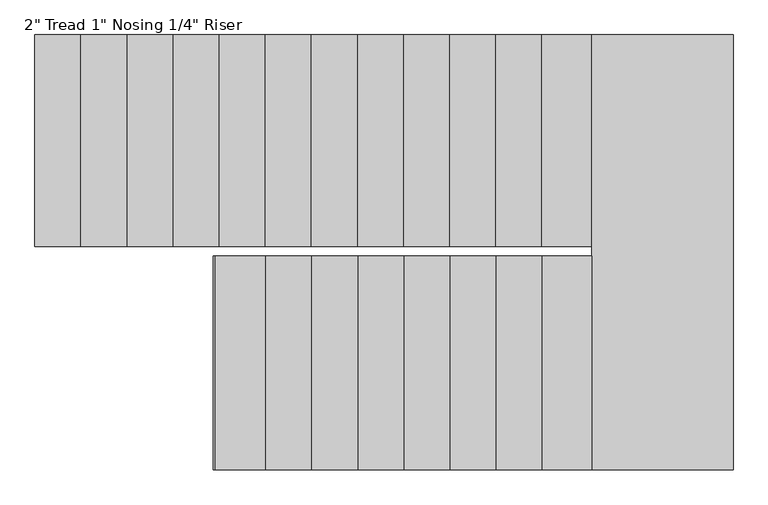
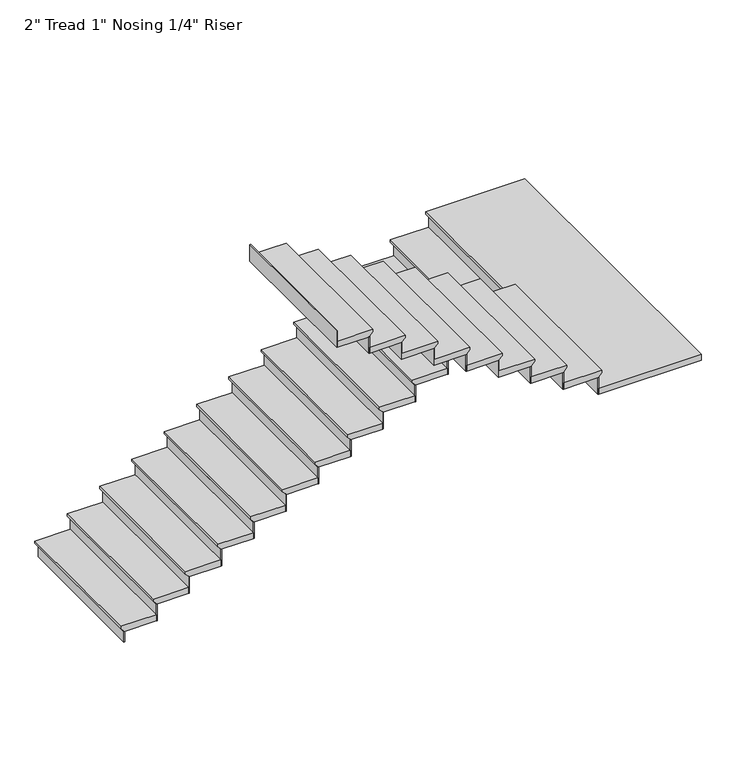
"""IFC4 building model written with IfcOpenShell, lengths in millimetres: stair flight geometry."""

from ifc_helpers import new_model, si_unit, origin, place, context, project, spatial, faceted_brep, source, transform, mapped, element, save


def stair_flight_e3e94c6b(model_context):
    return source(origin(), model_context, "Body", "Brep", [
        faceted_brep([(1811.8890963, 296.3962251, 3167.4954545), (1811.8890963, 296.3962251, 3186.5454545), (1811.8890963, 1464.7962251, 3186.5454545), (1811.8890963, 1464.7962251, 3167.4954545), (1837.2890963, 296.3962251, 3142.0954545), (1837.2890963, 1464.7962251, 3142.0954545), (2091.2890963, 296.3962251, 3186.5454545), (2091.2890963, 1464.7962251, 3186.5454545), (1837.2890963, 1464.7962251, 3135.7454545), (2091.2890963, 1464.7962251, 3135.7454545), (2091.2890963, 296.3962251, 3135.7454545), (1837.2890963, 296.3962251, 3135.7454545)], [[[0, 1, 2, 3]], [[4, 0, 3, 5]], [[2, 1, 6, 7]], [[8, 9, 10, 11]], [[2, 7, 9, 8, 5, 3]], [[8, 11, 4, 5]], [[6, 1, 0, 4, 11, 10]], [[7, 6, 10, 9]]]),
        faceted_brep([(1837.2890963, 296.3962251, 3135.7454545), (1837.2890963, 296.3962251, 3048.0), (1843.6390963, 296.3962251, 3048.0), (1843.6390963, 296.3962251, 3135.7454545), (1837.2890963, 1464.7962251, 3135.7454545), (1843.6390963, 1464.7962251, 3135.7454545), (1843.6390963, 1464.7962251, 3048.0), (1837.2890963, 1464.7962251, 3048.0)], [[[0, 1, 2, 3]], [[4, 5, 6, 7]], [[1, 0, 4, 7]], [[2, 1, 7, 6]], [[3, 2, 6, 5]], [[0, 3, 5, 4]]]),
        faceted_brep([(2091.2890963, 296.3962251, 3274.2909091), (2091.2890963, 296.3962251, 3135.7454545), (2097.6390963, 296.3962251, 3135.7454545), (2097.6390963, 296.3962251, 3274.2909091), (2091.2890963, 1464.7962251, 3274.2909091), (2097.6390963, 1464.7962251, 3274.2909091), (2097.6390963, 1464.7962251, 3135.7454545), (2091.2890963, 1464.7962251, 3135.7454545)], [[[0, 1, 2, 3]], [[4, 5, 6, 7]], [[1, 0, 4, 7]], [[2, 1, 7, 6]], [[3, 2, 6, 5]], [[0, 3, 5, 4]]]),
        faceted_brep([(2065.8890963, 1464.7962251, 3325.0909091), (2065.8890963, 296.3962251, 3325.0909091), (2345.2890963, 296.3962251, 3325.0909091), (2345.2890963, 1464.7962251, 3325.0909091), (2091.2890963, 1464.7962251, 3274.2909091), (2345.2890963, 1464.7962251, 3274.2909091), (2345.2890963, 296.3962251, 3274.2909091), (2091.2890963, 296.3962251, 3274.2909091), (2091.2890963, 1464.7962251, 3280.6409091), (2065.8890963, 1464.7962251, 3306.0409091), (2091.2890963, 296.3962251, 3280.6409091), (2065.8890963, 296.3962251, 3306.0409091)], [[[0, 1, 2, 3]], [[4, 5, 6, 7]], [[0, 3, 5, 4, 8, 9]], [[4, 7, 10, 8]], [[2, 1, 11, 10, 7, 6]], [[3, 2, 6, 5]], [[11, 1, 0, 9]], [[10, 11, 9, 8]]]),
        faceted_brep([(2345.2890963, 296.3962251, 3412.8363636), (2345.2890963, 296.3962251, 3274.2909091), (2351.6390963, 296.3962251, 3274.2909091), (2351.6390963, 296.3962251, 3412.8363636), (2345.2890963, 1464.7962251, 3412.8363636), (2351.6390963, 1464.7962251, 3412.8363636), (2351.6390963, 1464.7962251, 3274.2909091), (2345.2890963, 1464.7962251, 3274.2909091)], [[[0, 1, 2, 3]], [[4, 5, 6, 7]], [[1, 0, 4, 7]], [[2, 1, 7, 6]], [[3, 2, 6, 5]], [[0, 3, 5, 4]]]),
        faceted_brep([(2319.8890963, 1464.7962251, 3463.6363636), (2319.8890963, 296.3962251, 3463.6363636), (2599.2890963, 296.3962251, 3463.6363636), (2599.2890963, 1464.7962251, 3463.6363636), (2345.2890963, 1464.7962251, 3412.8363636), (2599.2890963, 1464.7962251, 3412.8363636), (2599.2890963, 296.3962251, 3412.8363636), (2345.2890963, 296.3962251, 3412.8363636), (2345.2890963, 1464.7962251, 3419.1863636), (2319.8890963, 1464.7962251, 3444.5863636), (2345.2890963, 296.3962251, 3419.1863636), (2319.8890963, 296.3962251, 3444.5863636)], [[[0, 1, 2, 3]], [[4, 5, 6, 7]], [[0, 3, 5, 4, 8, 9]], [[4, 7, 10, 8]], [[2, 1, 11, 10, 7, 6]], [[3, 2, 6, 5]], [[11, 1, 0, 9]], [[10, 11, 9, 8]]]),
        faceted_brep([(2599.2890963, 296.3962251, 3551.3818182), (2599.2890963, 296.3962251, 3412.8363636), (2605.6390963, 296.3962251, 3412.8363636), (2605.6390963, 296.3962251, 3551.3818182), (2599.2890963, 1464.7962251, 3551.3818182), (2605.6390963, 1464.7962251, 3551.3818182), (2605.6390963, 1464.7962251, 3412.8363636), (2599.2890963, 1464.7962251, 3412.8363636)], [[[0, 1, 2, 3]], [[4, 5, 6, 7]], [[1, 0, 4, 7]], [[2, 1, 7, 6]], [[3, 2, 6, 5]], [[0, 3, 5, 4]]]),
        faceted_brep([(2573.8890963, 1464.7962251, 3602.1818182), (2573.8890963, 296.3962251, 3602.1818182), (2853.2890963, 296.3962251, 3602.1818182), (2853.2890963, 1464.7962251, 3602.1818182), (2599.2890963, 1464.7962251, 3551.3818182), (2853.2890963, 1464.7962251, 3551.3818182), (2853.2890963, 296.3962251, 3551.3818182), (2599.2890963, 296.3962251, 3551.3818182), (2599.2890963, 1464.7962251, 3557.7318182), (2573.8890963, 1464.7962251, 3583.1318182), (2599.2890963, 296.3962251, 3557.7318182), (2573.8890963, 296.3962251, 3583.1318182)], [[[0, 1, 2, 3]], [[4, 5, 6, 7]], [[0, 3, 5, 4, 8, 9]], [[4, 7, 10, 8]], [[2, 1, 11, 10, 7, 6]], [[3, 2, 6, 5]], [[11, 1, 0, 9]], [[10, 11, 9, 8]]]),
        faceted_brep([(2853.2890963, 296.3962251, 3689.9272727), (2853.2890963, 296.3962251, 3551.3818182), (2859.6390963, 296.3962251, 3551.3818182), (2859.6390963, 296.3962251, 3689.9272727), (2853.2890963, 1464.7962251, 3689.9272727), (2859.6390963, 1464.7962251, 3689.9272727), (2859.6390963, 1464.7962251, 3551.3818182), (2853.2890963, 1464.7962251, 3551.3818182)], [[[0, 1, 2, 3]], [[4, 5, 6, 7]], [[1, 0, 4, 7]], [[2, 1, 7, 6]], [[3, 2, 6, 5]], [[0, 3, 5, 4]]]),
        faceted_brep([(2827.8890963, 1464.7962251, 3740.7272727), (2827.8890963, 296.3962251, 3740.7272727), (3107.2890963, 296.3962251, 3740.7272727), (3107.2890963, 1464.7962251, 3740.7272727), (2853.2890963, 1464.7962251, 3689.9272727), (3107.2890963, 1464.7962251, 3689.9272727), (3107.2890963, 296.3962251, 3689.9272727), (2853.2890963, 296.3962251, 3689.9272727), (2853.2890963, 1464.7962251, 3696.2772727), (2827.8890963, 1464.7962251, 3721.6772727), (2853.2890963, 296.3962251, 3696.2772727), (2827.8890963, 296.3962251, 3721.6772727)], [[[0, 1, 2, 3]], [[4, 5, 6, 7]], [[0, 3, 5, 4, 8, 9]], [[4, 7, 10, 8]], [[2, 1, 11, 10, 7, 6]], [[3, 2, 6, 5]], [[11, 1, 0, 9]], [[10, 11, 9, 8]]]),
        faceted_brep([(3107.2890963, 296.3962251, 3828.4727273), (3107.2890963, 296.3962251, 3689.9272727), (3113.6390963, 296.3962251, 3689.9272727), (3113.6390963, 296.3962251, 3828.4727273), (3107.2890963, 1464.7962251, 3828.4727273), (3113.6390963, 1464.7962251, 3828.4727273), (3113.6390963, 1464.7962251, 3689.9272727), (3107.2890963, 1464.7962251, 3689.9272727)], [[[0, 1, 2, 3]], [[4, 5, 6, 7]], [[1, 0, 4, 7]], [[2, 1, 7, 6]], [[3, 2, 6, 5]], [[0, 3, 5, 4]]]),
        faceted_brep([(3081.8890963, 1464.7962251, 3879.2727273), (3081.8890963, 296.3962251, 3879.2727273), (3361.2890963, 296.3962251, 3879.2727273), (3361.2890963, 1464.7962251, 3879.2727273), (3107.2890963, 1464.7962251, 3828.4727273), (3361.2890963, 1464.7962251, 3828.4727273), (3361.2890963, 296.3962251, 3828.4727273), (3107.2890963, 296.3962251, 3828.4727273), (3107.2890963, 1464.7962251, 3834.8227273), (3081.8890963, 1464.7962251, 3860.2227273), (3107.2890963, 296.3962251, 3834.8227273), (3081.8890963, 296.3962251, 3860.2227273)], [[[0, 1, 2, 3]], [[4, 5, 6, 7]], [[0, 3, 5, 4, 8, 9]], [[4, 7, 10, 8]], [[2, 1, 11, 10, 7, 6]], [[3, 2, 6, 5]], [[11, 1, 0, 9]], [[10, 11, 9, 8]]]),
        faceted_brep([(3361.2890963, 296.3962251, 3967.0181818), (3361.2890963, 296.3962251, 3828.4727273), (3367.6390963, 296.3962251, 3828.4727273), (3367.6390963, 296.3962251, 3967.0181818), (3361.2890963, 1464.7962251, 3967.0181818), (3367.6390963, 1464.7962251, 3967.0181818), (3367.6390963, 1464.7962251, 3828.4727273), (3361.2890963, 1464.7962251, 3828.4727273)], [[[0, 1, 2, 3]], [[4, 5, 6, 7]], [[1, 0, 4, 7]], [[2, 1, 7, 6]], [[3, 2, 6, 5]], [[0, 3, 5, 4]]]),
        faceted_brep([(3335.8890963, 1464.7962251, 4017.8181818), (3335.8890963, 296.3962251, 4017.8181818), (3615.2890963, 296.3962251, 4017.8181818), (3615.2890963, 1464.7962251, 4017.8181818), (3361.2890963, 1464.7962251, 3967.0181818), (3615.2890963, 1464.7962251, 3967.0181818), (3615.2890963, 296.3962251, 3967.0181818), (3361.2890963, 296.3962251, 3967.0181818), (3361.2890963, 1464.7962251, 3973.3681818), (3335.8890963, 1464.7962251, 3998.7681818), (3361.2890963, 296.3962251, 3973.3681818), (3335.8890963, 296.3962251, 3998.7681818)], [[[0, 1, 2, 3]], [[4, 5, 6, 7]], [[0, 3, 5, 4, 8, 9]], [[4, 7, 10, 8]], [[2, 1, 11, 10, 7, 6]], [[3, 2, 6, 5]], [[11, 1, 0, 9]], [[10, 11, 9, 8]]]),
        faceted_brep([(3615.2890963, 296.3962251, 4105.5636364), (3615.2890963, 296.3962251, 3967.0181818), (3621.6390963, 296.3962251, 3967.0181818), (3621.6390963, 296.3962251, 4105.5636364), (3615.2890963, 1464.7962251, 4105.5636364), (3621.6390963, 1464.7962251, 4105.5636364), (3621.6390963, 1464.7962251, 3967.0181818), (3615.2890963, 1464.7962251, 3967.0181818)], [[[0, 1, 2, 3]], [[4, 5, 6, 7]], [[1, 0, 4, 7]], [[2, 1, 7, 6]], [[3, 2, 6, 5]], [[0, 3, 5, 4]]]),
        faceted_brep([(3589.8890963, 1464.7962251, 4156.3636364), (3589.8890963, 296.3962251, 4156.3636364), (3869.2890963, 296.3962251, 4156.3636364), (3869.2890963, 1464.7962251, 4156.3636364), (3615.2890963, 1464.7962251, 4105.5636364), (3869.2890963, 1464.7962251, 4105.5636364), (3869.2890963, 296.3962251, 4105.5636364), (3615.2890963, 296.3962251, 4105.5636364), (3615.2890963, 1464.7962251, 4111.9136364), (3589.8890963, 1464.7962251, 4137.3136364), (3615.2890963, 296.3962251, 4111.9136364), (3589.8890963, 296.3962251, 4137.3136364)], [[[0, 1, 2, 3]], [[4, 5, 6, 7]], [[0, 3, 5, 4, 8, 9]], [[4, 7, 10, 8]], [[2, 1, 11, 10, 7, 6]], [[3, 2, 6, 5]], [[11, 1, 0, 9]], [[10, 11, 9, 8]]]),
        faceted_brep([(3869.2890963, 296.3962251, 4244.1090909), (3869.2890963, 296.3962251, 4105.5636364), (3875.6390963, 296.3962251, 4105.5636364), (3875.6390963, 296.3962251, 4244.1090909), (3869.2890963, 1464.7962251, 4244.1090909), (3875.6390963, 1464.7962251, 4244.1090909), (3875.6390963, 1464.7962251, 4105.5636364), (3869.2890963, 1464.7962251, 4105.5636364)], [[[0, 1, 2, 3]], [[4, 5, 6, 7]], [[1, 0, 4, 7]], [[2, 1, 7, 6]], [[3, 2, 6, 5]], [[0, 3, 5, 4]]]),
        faceted_brep([(3843.8890963, 1464.7962251, 4294.9090909), (3843.8890963, 296.3962251, 4294.9090909), (4123.2890963, 296.3962251, 4294.9090909), (4123.2890963, 1464.7962251, 4294.9090909), (3869.2890963, 1464.7962251, 4244.1090909), (4123.2890963, 1464.7962251, 4244.1090909), (4123.2890963, 296.3962251, 4244.1090909), (3869.2890963, 296.3962251, 4244.1090909), (3869.2890963, 1464.7962251, 4250.4590909), (3843.8890963, 1464.7962251, 4275.8590909), (3869.2890963, 296.3962251, 4250.4590909), (3843.8890963, 296.3962251, 4275.8590909)], [[[0, 1, 2, 3]], [[4, 5, 6, 7]], [[0, 3, 5, 4, 8, 9]], [[4, 7, 10, 8]], [[2, 1, 11, 10, 7, 6]], [[3, 2, 6, 5]], [[11, 1, 0, 9]], [[10, 11, 9, 8]]]),
        faceted_brep([(4123.2890963, 296.3962251, 4382.6545455), (4123.2890963, 296.3962251, 4244.1090909), (4129.6390963, 296.3962251, 4244.1090909), (4129.6390963, 296.3962251, 4382.6545455), (4123.2890963, 1464.7962251, 4382.6545455), (4129.6390963, 1464.7962251, 4382.6545455), (4129.6390963, 1464.7962251, 4244.1090909), (4123.2890963, 1464.7962251, 4244.1090909)], [[[0, 1, 2, 3]], [[4, 5, 6, 7]], [[1, 0, 4, 7]], [[2, 1, 7, 6]], [[3, 2, 6, 5]], [[0, 3, 5, 4]]]),
        faceted_brep([(4097.8890963, 1464.7962251, 4433.4545455), (4097.8890963, 296.3962251, 4433.4545455), (4377.2890963, 296.3962251, 4433.4545455), (4377.2890963, 1464.7962251, 4433.4545455), (4123.2890963, 1464.7962251, 4382.6545455), (4377.2890963, 1464.7962251, 4382.6545455), (4377.2890963, 296.3962251, 4382.6545455), (4123.2890963, 296.3962251, 4382.6545455), (4123.2890963, 1464.7962251, 4389.0045455), (4097.8890963, 1464.7962251, 4414.4045455), (4123.2890963, 296.3962251, 4389.0045455), (4097.8890963, 296.3962251, 4414.4045455)], [[[0, 1, 2, 3]], [[4, 5, 6, 7]], [[0, 3, 5, 4, 8, 9]], [[4, 7, 10, 8]], [[2, 1, 11, 10, 7, 6]], [[3, 2, 6, 5]], [[11, 1, 0, 9]], [[10, 11, 9, 8]]]),
        faceted_brep([(4377.2890963, 296.3962251, 4521.2), (4377.2890963, 296.3962251, 4382.6545455), (4383.6390963, 296.3962251, 4382.6545455), (4383.6390963, 296.3962251, 4521.2), (4377.2890963, 1464.7962251, 4521.2), (4383.6390963, 1464.7962251, 4521.2), (4383.6390963, 1464.7962251, 4382.6545455), (4377.2890963, 1464.7962251, 4382.6545455)], [[[0, 1, 2, 3]], [[4, 5, 6, 7]], [[1, 0, 4, 7]], [[2, 1, 7, 6]], [[3, 2, 6, 5]], [[0, 3, 5, 4]]]),
        faceted_brep([(4351.8890963, 1464.7962251, 4572.0), (4351.8890963, 296.3962251, 4572.0), (4631.2890963, 296.3962251, 4572.0), (4631.2890963, 1464.7962251, 4572.0), (4377.2890963, 1464.7962251, 4521.2), (4631.2890963, 1464.7962251, 4521.2), (4631.2890963, 296.3962251, 4521.2), (4377.2890963, 296.3962251, 4521.2), (4377.2890963, 1464.7962251, 4527.55), (4351.8890963, 1464.7962251, 4552.95), (4377.2890963, 296.3962251, 4527.55), (4351.8890963, 296.3962251, 4552.95)], [[[0, 1, 2, 3]], [[4, 5, 6, 7]], [[0, 3, 5, 4, 8, 9]], [[4, 7, 10, 8]], [[2, 1, 11, 10, 7, 6]], [[3, 2, 6, 5]], [[11, 1, 0, 9]], [[10, 11, 9, 8]]]),
        faceted_brep([(4631.2890963, 296.3962251, 4659.7454545), (4631.2890963, 296.3962251, 4521.2), (4637.6390963, 296.3962251, 4521.2), (4637.6390963, 296.3962251, 4659.7454545), (4631.2890963, 1464.7962251, 4659.7454545), (4637.6390963, 1464.7962251, 4659.7454545), (4637.6390963, 1464.7962251, 4521.2), (4631.2890963, 1464.7962251, 4521.2)], [[[0, 1, 2, 3]], [[4, 5, 6, 7]], [[1, 0, 4, 7]], [[2, 1, 7, 6]], [[3, 2, 6, 5]], [[0, 3, 5, 4]]]),
        faceted_brep([(4605.8890963, 1464.7962251, 4710.5454545), (4605.8890963, 296.3962251, 4710.5454545), (4906.4326586, 296.3962251, 4710.5454545), (4906.4326586, 1464.7962251, 4710.5454545), (4631.2890963, 1464.7962251, 4659.7454545), (4906.4326586, 1464.7962251, 4659.7454545), (4906.4326586, 296.3962251, 4659.7454545), (4631.2890963, 296.3962251, 4659.7454545), (4631.2890963, 1464.7962251, 4666.0954545), (4605.8890963, 1464.7962251, 4691.4954545), (4631.2890963, 296.3962251, 4666.0954545), (4605.8890963, 296.3962251, 4691.4954545)], [[[0, 1, 2, 3]], [[4, 5, 6, 7]], [[0, 3, 5, 4, 8, 9]], [[4, 7, 10, 8]], [[2, 1, 11, 10, 7, 6]], [[3, 2, 6, 5]], [[11, 1, 0, 9]], [[10, 11, 9, 8]]]),
        faceted_brep([(4906.4326586, 296.3962251, 4798.2909091), (4906.4326586, 296.3962251, 4659.7454545), (4912.7826586, 296.3962251, 4659.7454545), (4912.7826586, 296.3962251, 4798.2909091), (4906.4326586, 1464.7962251, 4798.2909091), (4912.7826586, 1464.7962251, 4798.2909091), (4912.7826586, 1464.7962251, 4659.7454545), (4906.4326586, 1464.7962251, 4659.7454545)], [[[0, 1, 2, 3]], [[4, 5, 6, 7]], [[1, 0, 4, 7]], [[2, 1, 7, 6]], [[3, 2, 6, 5]], [[0, 3, 5, 4]]]),
        faceted_brep([(4855.6326586, -935.5037749, 4849.0909091), (5659.9890963, -935.5037749, 4849.0909091), (5659.9890963, 1464.7962251, 4849.0909091), (4881.0326586, 1464.7962251, 4849.0909091), (4881.0326586, 245.5962251, 4849.0909091), (4855.6326586, 245.5962251, 4849.0909091), (5659.9890963, -935.5037749, 4798.2909091), (4855.6326586, -935.5037749, 4798.2909091), (4855.6326586, 245.5962251, 4798.2909091), (4881.0326586, 245.5962251, 4798.2909091), (4881.0326586, 296.3962251, 4798.2909091), (4906.4326586, 296.3962251, 4798.2909091), (4906.4326586, 1464.7962251, 4798.2909091), (5659.9890963, 1464.7962251, 4798.2909091), (4906.4326586, 1464.7962251, 4804.6409091), (4881.0326586, 1464.7962251, 4830.0409091), (4906.4326586, 296.3962251, 4804.6409091), (4881.0326586, 296.3962251, 4830.0409091)], [[[0, 1, 2, 3, 4, 5]], [[6, 7, 8, 9, 10, 11, 12, 13]], [[1, 0, 7, 6]], [[2, 1, 6, 13]], [[3, 2, 13, 12, 14, 15]], [[12, 11, 16, 14]], [[11, 10, 17, 16]], [[4, 3, 15, 17, 10, 9]], [[5, 4, 9, 8]], [[0, 5, 8, 7]], [[15, 14, 16, 17]]]),
        faceted_brep([(4855.6326586, 245.5962251, 4936.8363636), (4855.6326586, 245.5962251, 4798.2909091), (4849.2826586, 245.5962251, 4798.2909091), (4849.2826586, 245.5962251, 4936.8363636), (4855.6326586, -935.5037749, 4936.8363636), (4849.2826586, -935.5037749, 4936.8363636), (4849.2826586, -935.5037749, 4798.2909091), (4855.6326586, -935.5037749, 4798.2909091)], [[[0, 1, 2, 3]], [[4, 5, 6, 7]], [[1, 0, 4, 7]], [[2, 1, 7, 6]], [[3, 2, 6, 5]], [[0, 3, 5, 4]]]),
        faceted_brep([(4881.0326586, -935.5037749, 4987.6363636), (4881.0326586, 245.5962251, 4987.6363636), (4580.4890963, 245.5962251, 4987.6363636), (4580.4890963, -935.5037749, 4987.6363636), (4855.6326586, -935.5037749, 4936.8363636), (4580.4890963, -935.5037749, 4936.8363636), (4580.4890963, 245.5962251, 4936.8363636), (4855.6326586, 245.5962251, 4936.8363636), (4855.6326586, -935.5037749, 4943.1863636), (4881.0326586, -935.5037749, 4968.5863636), (4855.6326586, 245.5962251, 4943.1863636), (4881.0326586, 245.5962251, 4968.5863636)], [[[0, 1, 2, 3]], [[4, 5, 6, 7]], [[0, 3, 5, 4, 8, 9]], [[4, 7, 10, 8]], [[2, 1, 11, 10, 7, 6]], [[3, 2, 6, 5]], [[11, 1, 0, 9]], [[10, 11, 9, 8]]]),
        faceted_brep([(4580.4890963, 245.5962251, 5075.3818182), (4580.4890963, 245.5962251, 4936.8363636), (4574.1390963, 245.5962251, 4936.8363636), (4574.1390963, 245.5962251, 5075.3818182), (4580.4890963, -935.5037749, 5075.3818182), (4574.1390963, -935.5037749, 5075.3818182), (4574.1390963, -935.5037749, 4936.8363636), (4580.4890963, -935.5037749, 4936.8363636)], [[[0, 1, 2, 3]], [[4, 5, 6, 7]], [[1, 0, 4, 7]], [[2, 1, 7, 6]], [[3, 2, 6, 5]], [[0, 3, 5, 4]]]),
        faceted_brep([(4605.8890963, -935.5037749, 5126.1818182), (4605.8890963, 245.5962251, 5126.1818182), (4326.4890963, 245.5962251, 5126.1818182), (4326.4890963, -935.5037749, 5126.1818182), (4580.4890963, -935.5037749, 5075.3818182), (4326.4890963, -935.5037749, 5075.3818182), (4326.4890963, 245.5962251, 5075.3818182), (4580.4890963, 245.5962251, 5075.3818182), (4580.4890963, -935.5037749, 5081.7318182), (4605.8890963, -935.5037749, 5107.1318182), (4580.4890963, 245.5962251, 5081.7318182), (4605.8890963, 245.5962251, 5107.1318182)], [[[0, 1, 2, 3]], [[4, 5, 6, 7]], [[0, 3, 5, 4, 8, 9]], [[4, 7, 10, 8]], [[2, 1, 11, 10, 7, 6]], [[3, 2, 6, 5]], [[11, 1, 0, 9]], [[10, 11, 9, 8]]]),
        faceted_brep([(4326.4890963, 245.5962251, 5213.9272727), (4326.4890963, 245.5962251, 5075.3818182), (4320.1390963, 245.5962251, 5075.3818182), (4320.1390963, 245.5962251, 5213.9272727), (4326.4890963, -935.5037749, 5213.9272727), (4320.1390963, -935.5037749, 5213.9272727), (4320.1390963, -935.5037749, 5075.3818182), (4326.4890963, -935.5037749, 5075.3818182)], [[[0, 1, 2, 3]], [[4, 5, 6, 7]], [[1, 0, 4, 7]], [[2, 1, 7, 6]], [[3, 2, 6, 5]], [[0, 3, 5, 4]]]),
        faceted_brep([(4351.8890963, -935.5037749, 5264.7272727), (4351.8890963, 245.5962251, 5264.7272727), (4072.4890963, 245.5962251, 5264.7272727), (4072.4890963, -935.5037749, 5264.7272727), (4326.4890963, -935.5037749, 5213.9272727), (4072.4890963, -935.5037749, 5213.9272727), (4072.4890963, 245.5962251, 5213.9272727), (4326.4890963, 245.5962251, 5213.9272727), (4326.4890963, -935.5037749, 5220.2772727), (4351.8890963, -935.5037749, 5245.6772727), (4326.4890963, 245.5962251, 5220.2772727), (4351.8890963, 245.5962251, 5245.6772727)], [[[0, 1, 2, 3]], [[4, 5, 6, 7]], [[0, 3, 5, 4, 8, 9]], [[4, 7, 10, 8]], [[2, 1, 11, 10, 7, 6]], [[3, 2, 6, 5]], [[11, 1, 0, 9]], [[10, 11, 9, 8]]]),
        faceted_brep([(4072.4890963, 245.5962251, 5352.4727273), (4072.4890963, 245.5962251, 5213.9272727), (4066.1390963, 245.5962251, 5213.9272727), (4066.1390963, 245.5962251, 5352.4727273), (4072.4890963, -935.5037749, 5352.4727273), (4066.1390963, -935.5037749, 5352.4727273), (4066.1390963, -935.5037749, 5213.9272727), (4072.4890963, -935.5037749, 5213.9272727)], [[[0, 1, 2, 3]], [[4, 5, 6, 7]], [[1, 0, 4, 7]], [[2, 1, 7, 6]], [[3, 2, 6, 5]], [[0, 3, 5, 4]]]),
        faceted_brep([(4097.8890963, -935.5037749, 5403.2727273), (4097.8890963, 245.5962251, 5403.2727273), (3818.4890963, 245.5962251, 5403.2727273), (3818.4890963, -935.5037749, 5403.2727273), (4072.4890963, -935.5037749, 5352.4727273), (3818.4890963, -935.5037749, 5352.4727273), (3818.4890963, 245.5962251, 5352.4727273), (4072.4890963, 245.5962251, 5352.4727273), (4072.4890963, -935.5037749, 5358.8227273), (4097.8890963, -935.5037749, 5384.2227273), (4072.4890963, 245.5962251, 5358.8227273), (4097.8890963, 245.5962251, 5384.2227273)], [[[0, 1, 2, 3]], [[4, 5, 6, 7]], [[0, 3, 5, 4, 8, 9]], [[4, 7, 10, 8]], [[2, 1, 11, 10, 7, 6]], [[3, 2, 6, 5]], [[11, 1, 0, 9]], [[10, 11, 9, 8]]]),
        faceted_brep([(3818.4890963, 245.5962251, 5491.0181818), (3818.4890963, 245.5962251, 5352.4727273), (3812.1390963, 245.5962251, 5352.4727273), (3812.1390963, 245.5962251, 5491.0181818), (3818.4890963, -935.5037749, 5491.0181818), (3812.1390963, -935.5037749, 5491.0181818), (3812.1390963, -935.5037749, 5352.4727273), (3818.4890963, -935.5037749, 5352.4727273)], [[[0, 1, 2, 3]], [[4, 5, 6, 7]], [[1, 0, 4, 7]], [[2, 1, 7, 6]], [[3, 2, 6, 5]], [[0, 3, 5, 4]]]),
        faceted_brep([(3843.8890963, -935.5037749, 5541.8181818), (3843.8890963, 245.5962251, 5541.8181818), (3564.4890963, 245.5962251, 5541.8181818), (3564.4890963, -935.5037749, 5541.8181818), (3818.4890963, -935.5037749, 5491.0181818), (3564.4890963, -935.5037749, 5491.0181818), (3564.4890963, 245.5962251, 5491.0181818), (3818.4890963, 245.5962251, 5491.0181818), (3818.4890963, -935.5037749, 5497.3681818), (3843.8890963, -935.5037749, 5522.7681818), (3818.4890963, 245.5962251, 5497.3681818), (3843.8890963, 245.5962251, 5522.7681818)], [[[0, 1, 2, 3]], [[4, 5, 6, 7]], [[0, 3, 5, 4, 8, 9]], [[4, 7, 10, 8]], [[2, 1, 11, 10, 7, 6]], [[3, 2, 6, 5]], [[11, 1, 0, 9]], [[10, 11, 9, 8]]]),
        faceted_brep([(3564.4890963, 245.5962251, 5629.5636364), (3564.4890963, 245.5962251, 5491.0181818), (3558.1390963, 245.5962251, 5491.0181818), (3558.1390963, 245.5962251, 5629.5636364), (3564.4890963, -935.5037749, 5629.5636364), (3558.1390963, -935.5037749, 5629.5636364), (3558.1390963, -935.5037749, 5491.0181818), (3564.4890963, -935.5037749, 5491.0181818)], [[[0, 1, 2, 3]], [[4, 5, 6, 7]], [[1, 0, 4, 7]], [[2, 1, 7, 6]], [[3, 2, 6, 5]], [[0, 3, 5, 4]]]),
        faceted_brep([(3589.8890963, -935.5037749, 5680.3636364), (3589.8890963, 245.5962251, 5680.3636364), (3310.4890963, 245.5962251, 5680.3636364), (3310.4890963, -935.5037749, 5680.3636364), (3564.4890963, -935.5037749, 5629.5636364), (3310.4890963, -935.5037749, 5629.5636364), (3310.4890963, 245.5962251, 5629.5636364), (3564.4890963, 245.5962251, 5629.5636364), (3564.4890963, -935.5037749, 5635.9136364), (3589.8890963, -935.5037749, 5661.3136364), (3564.4890963, 245.5962251, 5635.9136364), (3589.8890963, 245.5962251, 5661.3136364)], [[[0, 1, 2, 3]], [[4, 5, 6, 7]], [[0, 3, 5, 4, 8, 9]], [[4, 7, 10, 8]], [[2, 1, 11, 10, 7, 6]], [[3, 2, 6, 5]], [[11, 1, 0, 9]], [[10, 11, 9, 8]]]),
        faceted_brep([(3310.4890963, 245.5962251, 5768.1090909), (3310.4890963, 245.5962251, 5629.5636364), (3304.1390963, 245.5962251, 5629.5636364), (3304.1390963, 245.5962251, 5768.1090909), (3310.4890963, -935.5037749, 5768.1090909), (3304.1390963, -935.5037749, 5768.1090909), (3304.1390963, -935.5037749, 5629.5636364), (3310.4890963, -935.5037749, 5629.5636364)], [[[0, 1, 2, 3]], [[4, 5, 6, 7]], [[1, 0, 4, 7]], [[2, 1, 7, 6]], [[3, 2, 6, 5]], [[0, 3, 5, 4]]]),
        faceted_brep([(3335.8890963, -935.5037749, 5818.9090909), (3335.8890963, 245.5962251, 5818.9090909), (3056.4890963, 245.5962251, 5818.9090909), (3056.4890963, -935.5037749, 5818.9090909), (3310.4890963, -935.5037749, 5768.1090909), (3056.4890963, -935.5037749, 5768.1090909), (3056.4890963, 245.5962251, 5768.1090909), (3310.4890963, 245.5962251, 5768.1090909), (3310.4890963, -935.5037749, 5774.4590909), (3335.8890963, -935.5037749, 5799.8590909), (3310.4890963, 245.5962251, 5774.4590909), (3335.8890963, 245.5962251, 5799.8590909)], [[[0, 1, 2, 3]], [[4, 5, 6, 7]], [[0, 3, 5, 4, 8, 9]], [[4, 7, 10, 8]], [[2, 1, 11, 10, 7, 6]], [[3, 2, 6, 5]], [[11, 1, 0, 9]], [[10, 11, 9, 8]]]),
        faceted_brep([(3056.4890963, 245.5962251, 5906.6545455), (3056.4890963, 245.5962251, 5768.1090909), (3050.1390963, 245.5962251, 5768.1090909), (3050.1390963, 245.5962251, 5906.6545455), (3056.4890963, -935.5037749, 5906.6545455), (3050.1390963, -935.5037749, 5906.6545455), (3050.1390963, -935.5037749, 5768.1090909), (3056.4890963, -935.5037749, 5768.1090909)], [[[0, 1, 2, 3]], [[4, 5, 6, 7]], [[1, 0, 4, 7]], [[2, 1, 7, 6]], [[3, 2, 6, 5]], [[0, 3, 5, 4]]]),
        faceted_brep([(2802.4890963, 245.5962251, 6045.2), (2802.4890963, 245.5962251, 5906.6545455), (2796.1390963, 245.5962251, 5906.6545455), (2796.1390963, 245.5962251, 6045.2), (2802.4890963, -935.5037749, 6045.2), (2796.1390963, -935.5037749, 6045.2), (2796.1390963, -935.5037749, 5906.6545455), (2802.4890963, -935.5037749, 5906.6545455)], [[[0, 1, 2, 3]], [[4, 5, 6, 7]], [[1, 0, 4, 7]], [[2, 1, 7, 6]], [[3, 2, 6, 5]], [[0, 3, 5, 4]]]),
        faceted_brep([(3081.8890963, -935.5037749, 5957.4545455), (3081.8890963, 245.5962251, 5957.4545455), (2802.4890963, 245.5962251, 5957.4545455), (2802.4890963, -935.5037749, 5957.4545455), (3056.4890963, -935.5037749, 5906.6545455), (2802.4890963, -935.5037749, 5906.6545455), (2802.4890963, 245.5962251, 5906.6545455), (3056.4890963, 245.5962251, 5906.6545455), (3056.4890963, -935.5037749, 5913.0045455), (3081.8890963, -935.5037749, 5938.4045455), (3056.4890963, 245.5962251, 5913.0045455), (3081.8890963, 245.5962251, 5938.4045455)], [[[0, 1, 2, 3]], [[4, 5, 6, 7]], [[0, 3, 5, 4, 8, 9]], [[4, 7, 10, 8]], [[2, 1, 11, 10, 7, 6]], [[3, 2, 6, 5]], [[11, 1, 0, 9]], [[10, 11, 9, 8]]]),
    ])


if __name__ == "__main__":
    model = new_model("IFC4")
    model_context = context("Model", 3, world=origin())
    ifc_project = project(units=[si_unit("LENGTHUNIT", "METRE", prefix="MILLI")], contexts=[model_context])
    site = spatial("IfcSite", under=ifc_project)
    building = spatial("IfcBuilding", under=site)
    placement = place(None, origin())
    stair_flight_shape = stair_flight_e3e94c6b(model_context)
    element("IfcStairFlight", 1, ObjectType="2\" Tread 1\" Nosing 1/4\" Riser", at=placement, inside=building, context=model_context, shape_type="MappedRepresentation", body=[
        mapped(stair_flight_shape, transform((0.0, 0.0, 0.0), x_axis=(1.0, 0.0, 0.0), y_axis=(0.0, 1.0, 0.0), z_axis=(0.0, 0.0, 1.0))),
    ])
    save(model, "model.ifc")
